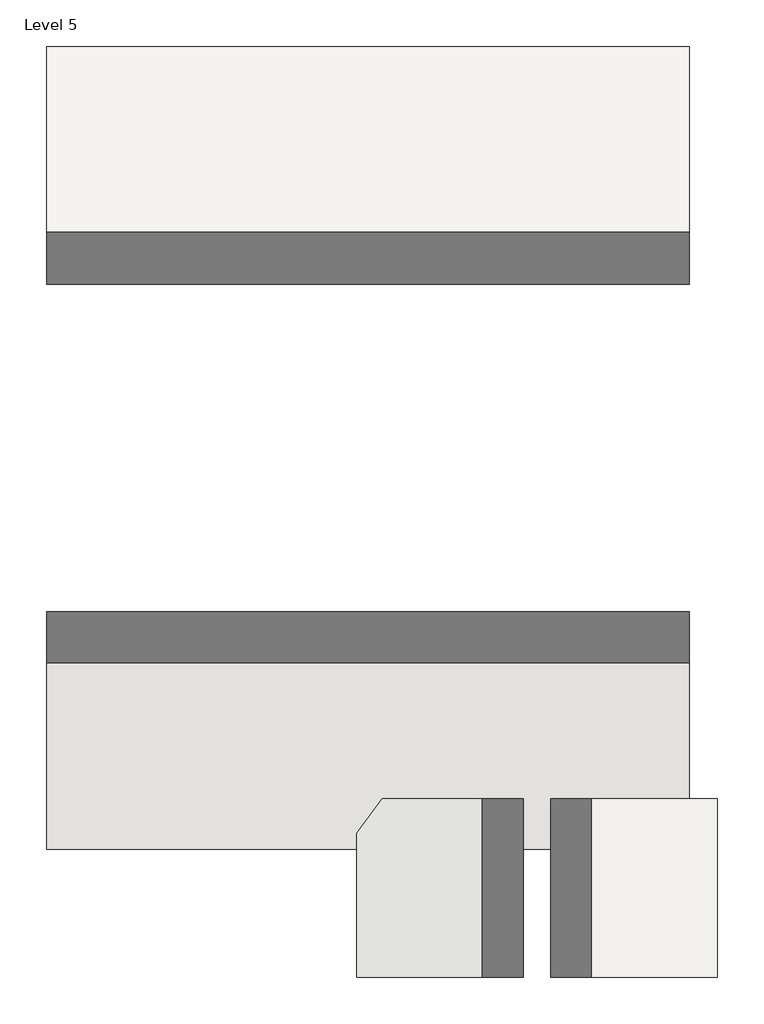
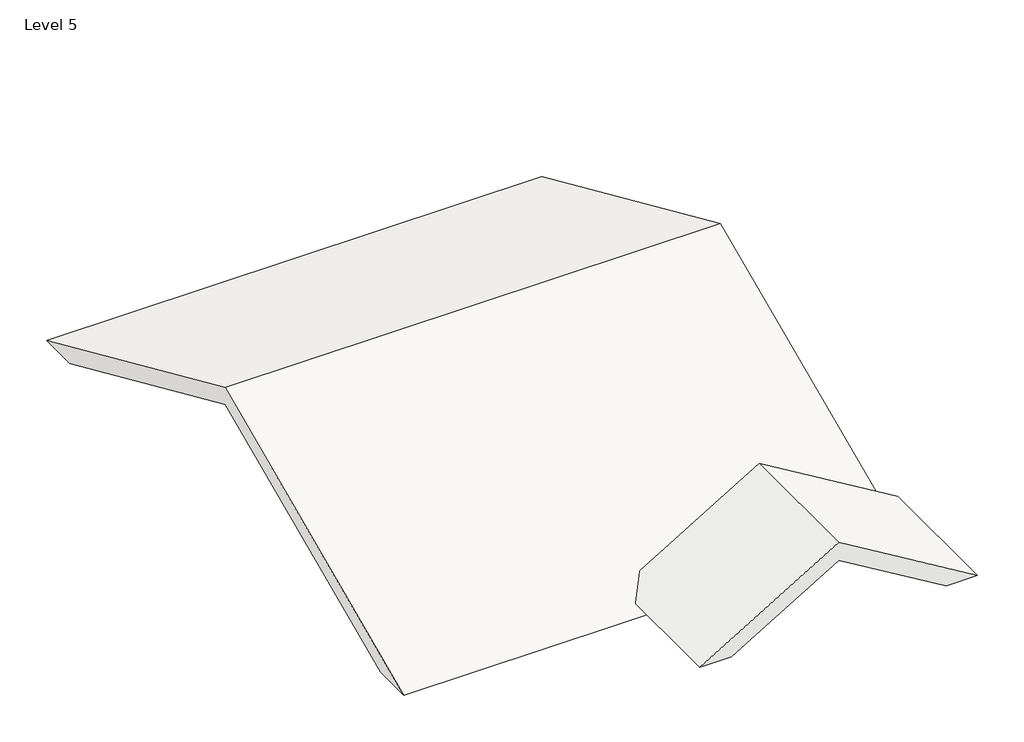
# One storey: 2 roofs.
"""IFC4 building model written with IfcOpenShell, lengths in millimetres."""

from ifc_helpers import new_model, si_unit, frame, origin, place, context, project, spatial, polyline, outline, extrude, element, save

model = new_model("IFC4")

# Units and contexts
model_context = context("Model", 3, world=origin())
ifc_project = project(units=[si_unit("LENGTHUNIT", "METRE", prefix="MILLI")], contexts=[model_context])

# Site, building, storey
site = spatial("IfcSite", under=ifc_project)
building = spatial("IfcBuilding", under=site)
storey = spatial("IfcBuildingStorey", under=building, Name="Level 5", Elevation=8077.2)

# Roofs
placement = place(None, origin())
element("IfcRoof", 1, ObjectType="Generic - 12\"", at=placement, inside=storey, context=model_context, shape_type="SweptSolid", body=[
    extrude(outline(polyline([(9753.6, 5347.8135732), (8183.7639477, 2735.1676407), (8183.7639477, 3326.968548), (9398.0101405, 5347.8135732), (8183.7639477, 7368.6585985), (8183.7639477, 7960.4595058), (9753.6, 5347.8135732)])), frame((0.0, -1733.1234736, 0.0), z_axis=(0.0, 1.0, 0.0), x_axis=(0.0, 0.0, 1.0)), (0.0, 0.0, 1.0), 2590.4157954),
])
element("IfcRoof", 2, ObjectType="Generic - 12\"", at=placement, inside=storey, context=model_context, shape_type="SweptSolid", body=[
    extrude(outline(polyline([(5944.0265264, 10668.0), (11763.0586002, 8077.2), (11013.6793515, 8077.2), (5944.0265264, 10334.3548623), (874.3737012, 8077.2), (124.9944526, 8077.2), (5944.0265264, 10668.0)])), frame((-1763.2651673, 0.0, 0.0), z_axis=(1.0, 0.0, 0.0), x_axis=(0.0, 1.0, 0.0)), (0.0, 0.0, 1.0), 9320.8787406),
])

save(model, "model.ifc")

# Revit data of these elements
# Type "Generic - 12\""
#   Assembly Code = "B1020"
#   Layers, outside or top first: 1' - 0" "roof" (function 1)
# Elements 1, 2 (IfcRoof, "Generic - 12\"")
#   built-in parameter 1001710 = 33619
#   Phase Created = New Construction
#   Materials on its faces: "roof"
# Materials
#   "roof": class "Generic", colour RGB 120 120 120, transparency 0, Cost = 0
